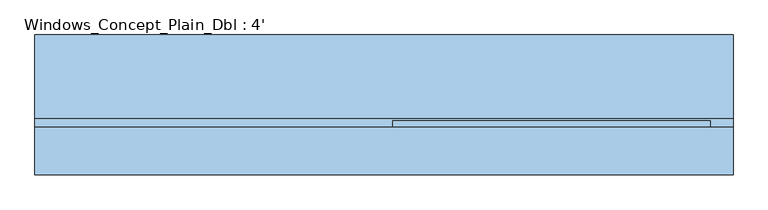
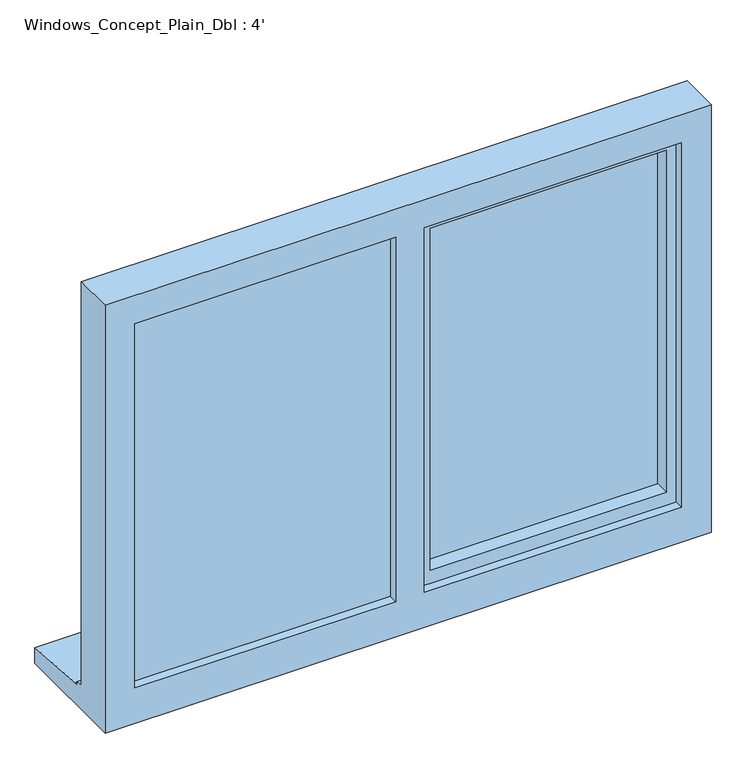
"""IFC4 building model written with IfcOpenShell, lengths in millimetres: window geometry, Windows_Concept_Plain_Dbl : 4'."""

from ifc_helpers import new_model, si_unit, frame, origin, place, context, project, spatial, polyline, outline, extrude, faceted_brep, source, transform, mapped, element, save


def windows_concept_plain_dbl_4_d1e2e333(model_context):
    return source(origin(), model_context, "Body", "SolidModel", [
        faceted_brep([(-270.0, -30.3434322, 2070.0), (-270.0, 46.2035732, 2070.0), (-270.0, 46.2035732, 1263.0), (-270.0, -30.3434322, 1263.0), (-230.0, -1.3434322, 2030.0), (-230.0, -30.3434322, 2030.0), (-230.0, -30.3434322, 1303.0), (-230.0, -1.3434322, 1303.0), (-240.0, 22.6565678, 2040.0), (-240.0, -1.3434322, 2040.0), (-240.0, -1.3434322, 1293.0), (-240.0, 22.6565678, 1293.0), (-230.0, 46.2035732, 2030.0), (-230.0, 22.6565678, 2030.0), (-230.0, 22.6565678, 1303.0), (-230.0, 46.2035732, 1303.0), (284.6, 46.2035732, 1263.0), (284.6, -30.3434322, 1263.0), (244.6, -30.3434322, 1303.0), (244.6, -1.3434322, 1303.0), (254.6, -1.3434322, 1293.0), (254.6, 22.6565678, 1293.0), (244.6, 22.6565678, 1303.0), (244.6, 46.2035732, 1303.0), (284.6, 46.2035732, 2070.0), (284.6, -30.3434322, 2070.0), (244.6, -30.3434322, 2030.0), (244.6, -1.3434322, 2030.0), (254.6, -1.3434322, 2040.0), (254.6, 22.6565678, 2040.0), (244.6, 22.6565678, 2030.0), (244.6, 46.2035732, 2030.0)], [[[0, 1, 2, 3]], [[4, 5, 6, 7]], [[8, 9, 10, 11]], [[12, 13, 14, 15]], [[3, 2, 16, 17]], [[7, 6, 18, 19]], [[11, 10, 20, 21]], [[15, 14, 22, 23]], [[17, 16, 24, 25]], [[19, 18, 26, 27]], [[21, 20, 28, 29]], [[23, 22, 30, 31]], [[1, 24, 16, 2], [15, 23, 31, 12]], [[25, 24, 1, 0]], [[3, 17, 25, 0], [5, 26, 18, 6]], [[27, 26, 5, 4]], [[9, 28, 20, 10], [7, 19, 27, 4]], [[29, 28, 9, 8]], [[11, 21, 29, 8], [13, 30, 22, 14]], [[31, 30, 13, 12]]]),
        extrude(outline(polyline([(2050.0, -310.0), (2070.0, -310.0), (2070.0, -854.6), (1263.0, -854.6), (1263.0, -310.0), (1283.0, -310.0), (1283.0, -834.6), (2050.0, -834.6), (2050.0, -310.0)])), frame((0.0, -6.3434322, 0.0), z_axis=(0.0, 1.0, 0.0), x_axis=(0.0, 0.0, 1.0)), (0.0, 0.0, 1.0), 41.0),
        faceted_brep([(324.6, -48.3434322, 2110.0), (-894.6, -48.3434322, 2110.0), (-894.6, -48.3434322, 1200.0), (324.6, -48.3434322, 1200.0), (264.6, -48.3434322, 2050.0), (264.6, -48.3434322, 1275.0), (-252.0, -48.3434322, 1275.0), (-252.0, -48.3434322, 2050.0), (-310.0, -48.3434322, 2050.0), (-310.0, -48.3434322, 1275.0), (-834.6, -48.3434322, 1275.0), (-834.6, -48.3434322, 2050.0), (-894.6, 34.6565678, 2110.0), (-894.6, 34.6565678, 1251.0), (-894.6, 49.6565678, 1249.68767), (-894.6, 49.6565678, 1244.7449676), (-894.6, 195.9565678, 1233.8088847), (-894.6, 195.9565678, 1200.0), (324.6, 34.6565678, 2110.0), (324.6, 34.6565678, 1251.0), (-854.6, 34.6565678, 2070.0), (-854.6, 34.6565678, 1263.0), (-310.0, 34.6565678, 1263.0), (-310.0, 34.6565678, 2070.0), (-270.0, 34.6565678, 2070.0), (-270.0, 34.6565678, 1263.0), (284.6, 34.6565678, 1263.0), (284.6, 34.6565678, 2070.0), (-854.6, -30.3434322, 2070.0), (-854.6, -30.3434322, 1263.0), (-300.0, -30.3434322, 2070.0), (-300.0, -30.3434322, 1263.0), (-310.0, -30.3434322, 2050.0), (-834.6, -30.3434322, 2050.0), (-834.6, -30.3434322, 1275.0), (-310.0, -30.3434322, 1275.0), (-270.0, -30.3434322, 2070.0), (284.6, -30.3434322, 2070.0), (284.6, -30.3434322, 1263.0), (-270.0, -30.3434322, 1263.0), (264.6, -30.3434322, 2050.0), (-252.0, -30.3434322, 2050.0), (-252.0, -30.3434322, 1275.0), (264.6, -30.3434322, 1275.0), (-310.0, -6.3434322, 2070.0), (-300.0, -6.3434322, 2070.0), (324.6, 195.9565678, 1200.0), (324.6, 195.9565678, 1233.8088847), (324.6, 49.6565678, 1244.7449676), (324.6, 49.6565678, 1249.68767), (-300.0, -6.3434322, 1263.0), (-310.0, -6.3434322, 1263.0)], [[[0, 1, 2, 3], [4, 5, 6, 7], [8, 9, 10, 11]], [[2, 1, 12, 13, 14, 15, 16, 17]], [[13, 12, 18, 19], [20, 21, 22, 23], [24, 25, 26, 27]], [[21, 20, 28, 29]], [[28, 30, 31, 29], [32, 33, 34, 35]], [[36, 37, 38, 39], [40, 41, 42, 43]], [[33, 11, 10, 34]], [[1, 0, 18, 12]], [[28, 20, 23, 44, 45, 30]], [[27, 37, 36, 24]], [[11, 33, 32, 8]], [[40, 4, 7, 41]], [[19, 18, 0, 3, 46, 47, 48, 49]], [[27, 26, 38, 37]], [[4, 40, 43, 5]], [[45, 50, 31, 30]], [[50, 45, 44, 51]], [[51, 44, 23, 22]], [[25, 24, 36, 39]], [[41, 7, 6, 42]], [[8, 32, 35, 9]], [[46, 3, 2, 17]], [[47, 46, 17, 16]], [[48, 47, 16, 15]], [[49, 48, 15, 14]], [[19, 49, 14, 13]], [[22, 21, 29, 31, 50, 51]], [[26, 25, 39, 38]], [[6, 5, 43, 42]], [[35, 34, 10, 9]]]),
        extrude(outline(polyline([(-854.6, -6.3434322), (-300.0, -6.3434322), (-300.0, -30.3434322), (-854.6, -30.3434322), (-854.6, -6.3434322)])), frame((0.0, 0.0, 1263.0), z_axis=(0.0, 0.0, 1.0), x_axis=(1.0, 0.0, 0.0)), (0.0, 0.0, 1.0), 807.0),
        extrude(outline(polyline([(254.6, -1.3434322), (-240.0, -1.3434322), (-240.0, 22.6565678), (254.6, 22.6565678), (254.6, -1.3434322)])), frame((0.0, 0.0, 1293.0), z_axis=(0.0, 0.0, 1.0), x_axis=(1.0, 0.0, 0.0)), (0.0, 0.0, 1.0), 747.0),
    ])


if __name__ == "__main__":
    model = new_model("IFC4")
    model_context = context("Model", 3, world=origin())
    ifc_project = project(units=[si_unit("LENGTHUNIT", "METRE", prefix="MILLI")], contexts=[model_context])
    site = spatial("IfcSite", under=ifc_project)
    building = spatial("IfcBuilding", under=site)
    placement = place(None, origin())
    windows_concept_plain_dbl_4_shape = windows_concept_plain_dbl_4_d1e2e333(model_context)
    element("IfcWindow", 1, ObjectType="Windows_Concept_Plain_Dbl : 4'", at=placement, inside=building, context=model_context, shape_type="MappedRepresentation", body=[
        mapped(windows_concept_plain_dbl_4_shape, transform((0.0, 0.0, 0.0), x_axis=(1.0, 0.0, 0.0), y_axis=(0.0, 1.0, 0.0), z_axis=(0.0, 0.0, 1.0))),
    ])
    save(model, "model.ifc")

# Revit data of these elements
# Type "Windows_Concept_Plain_Dbl : 4'"
#   Type Mark = "56"
#   Operation = "DoublePanelVertical"
#   Construction Type Id = "GSP4R"
#   Manufacturer = "Revit"
#   Keynote = "L10"
#   Analytic Construction = "1/8 in Pilkington single glazing"
#   Visual Light Transmittance = 0.9
#   Solar Heat Gain Coefficient = 0.78
#   Rough Width = 1219.2 mm
#   Rough Height = 910 mm
#   Height = 910 mm
#   Width = 1219.2 mm
#   Heat Transfer Coefficient (U) = 3.6886 W/(m²·K)
#   FrameOffset - External = 50 mm
#   Default Head Height = 2110 mm
#   Vis - Cavity Closers = yes
#   Define Thermal Properties by = 1
#   Material Trim = Window Frame
#   Material Glass = Glass
#   Material Frame = Window Frame
#   Wall Closure = (empty or 0)
# Element 1 (IfcWindow, "Windows_Concept_Plain_Dbl : 4'")
#   Materials on its faces: "Window Frame", "Glass"
# Materials
#   "Window Frame": colour RGB 249 249 249, transparency 0, Keynote = "L10", Cost = 0
#   "Glass": class "Glass", colour RGB 0 128 192, transparency 0.9, Description = "Soda Lime Glass", Cost = 0
